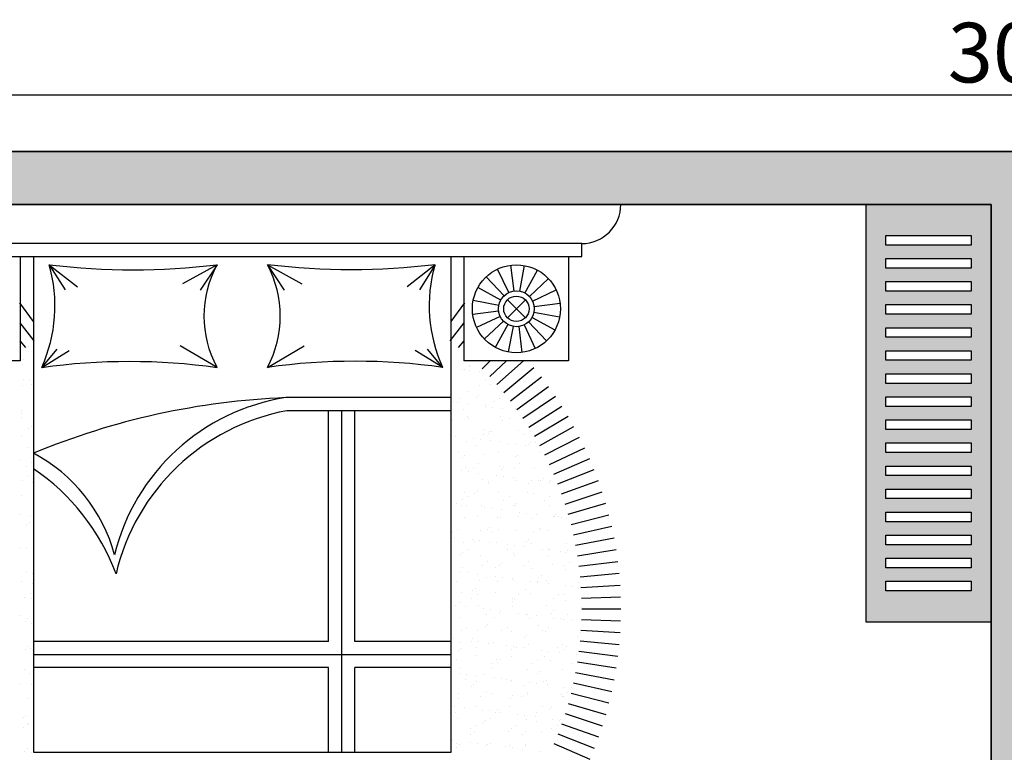
# Model space of a CAD drawing. Units: inches. Extents: x 1566 to 2546, y 1087 to 2705.
# Tile 22 of 27: x 2130 to 2278, y 1694 to 1804. Entities that reach past the tile are written whole.
import ezdxf

# ---------------------------------------------------------------- set-up
doc = ezdxf.new("R2010")
doc.units = ezdxf.units.IN
for name, color, linetype, lineweight in [('A-ANNO-DIMS', 2, 'Continuous', 18), ('A-FURN', 8, 'Continuous', 18), ('A-WALL', 7, 'Continuous', 35), ('A-WALL-PATT', 8, 'Continuous', 13)]:
    doc.layers.add(name, color=color, linetype=linetype, lineweight=lineweight)
for name, color, linetype in [('A-FRN', 11, 'Continuous'), ('A-HT', 15, 'Continuous'), ('L-HT', 1, 'Continuous'), ('MESA', 7, 'Continuous')]:
    doc.layers.add(name, color=color, linetype=linetype)
doc.styles.get("Standard").update_dxf_attribs({"font": 'arial.ttf'})
doc.dimstyles.new('ISO-25', dxfattribs={"dimtxt": 2.5, "dimasz": 2.5, "dimexe": 1.25, "dimexo": 0.625, "dimtad": 1, "dimtxsty": 'Standard', "dimcen": 2.5, "dimadec": 0, "dimazin": 0, "dimtfac": 1, "dimtmove": 0, "dimatfit": 3, "dimfxl": 1, "dimarcsym": 0})

# ---------------------------------------------------------------- blocks, each defined once
blk = doc.blocks.new('*D2')
at = {"layer": 'A-ANNO-DIMS', "color": 0, "lineweight": -2, "transparency": 16777216}
for p, q in [((2098.29, 1785.06), (2098.29, 1794.2)), ((2458.29, 1785.06), (2458.29, 1794.2)), ((2100.79, 1792.95), (2455.79, 1792.95))]:
    blk.add_line(p, q, dxfattribs=at)
at = {"layer": 'A-ANNO-DIMS', "color": 0, "transparency": 16777216}
for points in [[(2100.79, 1793.37), (2100.79, 1792.53), (2098.29, 1792.95)], [(2455.79, 1793.37), (2455.79, 1792.53), (2458.29, 1792.95)]]:
    blk.add_solid(points, dxfattribs=at)
at = {"layer": 'Defpoints', "color": 0, "transparency": 16777216}
for p in [(2458.29, 1792.95), (2098.29, 1784.43), (2458.29, 1784.43)]:
    blk.add_point(p, dxfattribs=at)
at = {"layer": 'A-ANNO-DIMS', "color": 0, "transparency": 16777216, "insert": (2278.29, 1798.17), "char_height": 9, "attachment_point": 5}
blk.add_mtext("30'", dxfattribs=at)
blk = doc.blocks.new('*X21')
at = {"color": 0}
for p, q in [((1.1667, 2.0955), (1.1667, 2.0955)), ((1.1756, 2.0872), (1.1756, 2.0872)), ((1.1927, 2.0989), (1.1927, 2.0989)), ((2.8216, 2.08), (2.8216, 2.08)), ((3.0086, 2.079), (3.0086, 2.079)), ((3.0247, 2.0756), (3.0247, 2.0756)), ((3.0346, 2.0825), (3.0346, 2.0825)), ((3.0752, 2.0878), (3.0752, 2.0878)), ((3.1432, 2.0968), (3.1432, 2.0968)), ((2.8061, 2.0524), (2.8061, 2.0524)), ((2.8215, 2.0663), (2.8215, 2.0663)), ((2.8309, 2.0716), (2.8309, 2.0716)), ((2.874, 2.0613), (2.874, 2.0613)), ((2.9, 2.0647), (2.9, 2.0647)), ((2.9303, 2.0732), (2.9303, 2.0732)), ((2.9407, 2.0701), (2.9407, 2.0701)), ((2.9494, 2.0657), (2.9494, 2.0657)), ((3.0845, 2.0705), (3.0845, 2.0705)), ((3.086, 2.0735), (3.086, 2.0735)), ((1.1609, 2.0067), (1.1609, 2.0067)), ((2.8737, 2.0098), (2.8737, 2.0098)), ((2.8744, 2.0317), (2.8744, 2.0317)), ((2.8891, 2.0194), (2.8891, 2.0194)), ((3.02, 2.0211), (3.02, 2.0211)), ((3.0294, 2.0101), (3.0294, 2.0101)), ((3.0744, 2.03), (3.0744, 2.03)), ((3.0837, 2.0216), (3.0837, 2.0216)), ((3.1479, 2.0205), (3.1479, 2.0205)), ((3.1851, 2.0104), (3.1851, 2.0104)), ((1.1614, 1.9668), (1.1614, 1.9668)), ((1.1788, 1.9909), (1.1788, 1.9909)), ((1.182, 1.9932), (1.182, 1.9932)), ((2.8247, 1.9699), (2.8247, 1.9699)), ((2.8947, 1.9964), (2.8947, 1.9964)), ((2.9241, 1.9861), (2.9241, 1.9861)), ((2.9333, 1.9777), (2.9333, 1.9777)), ((2.9526, 1.9693), (2.9526, 1.9693)), ((3.0505, 1.9966), (3.0505, 1.9966)), ((3.0876, 1.9742), (3.0876, 1.9742)), ((3.1213, 1.9644), (3.1213, 1.9644)), ((3.1272, 1.9817), (3.1272, 1.9817)), ((3.1893, 1.9734), (3.1893, 1.9734)), ((3.2062, 1.9969), (3.2062, 1.9969)), ((3.2153, 1.9768), (3.2153, 1.9768)), ((3.2185, 1.9759), (3.2185, 1.9759)), ((1.1707, 1.9584), (1.1707, 1.9584)), ((2.8115, 1.9236), (2.8115, 1.9236)), ((2.8149, 1.9477), (2.8149, 1.9477)), ((2.8522, 1.929), (2.8522, 1.929)), ((2.9201, 1.9379), (2.9201, 1.9379)), ((2.9461, 1.9414), (2.9461, 1.9414)), ((2.9707, 1.948), (2.9707, 1.948)), ((2.9768, 1.9378), (2.9768, 1.9378)), ((2.9868, 1.9467), (2.9868, 1.9467)), ((3.0232, 1.9247), (3.0232, 1.9247)), ((3.0547, 1.9556), (3.0547, 1.9556)), ((3.0807, 1.9591), (3.0807, 1.9591)), ((3.1264, 1.9483), (3.1264, 1.9483)), ((3.1511, 1.9241), (3.1511, 1.9241)), ((3.1769, 1.9361), (3.1769, 1.9361)), ((3.1861, 1.9277), (3.1861, 1.9277)), ((1.1819, 1.8945), (1.1819, 1.8945)), ((2.8265, 1.894), (2.8265, 1.894)), ((2.8923, 1.9231), (2.8923, 1.9231)), ((3.0266, 1.8922), (3.0266, 1.8922)), ((3.2296, 1.8878), (3.2296, 1.8878)), ((2.8278, 1.8736), (2.8278, 1.8736)), ((2.8763, 1.8484), (2.8763, 1.8484)), ((2.914, 1.8846), (2.914, 1.8846)), ((2.9351, 1.8712), (2.9351, 1.8712)), ((2.9557, 1.873), (2.9557, 1.873)), ((3.0358, 1.8838), (3.0358, 1.8838)), ((3.0697, 1.8849), (3.0697, 1.8849)), ((3.0908, 1.8779), (3.0908, 1.8779)), ((3.0908, 1.8714), (3.0908, 1.8714)), ((3.2217, 1.8795), (3.2217, 1.8795)), ((3.2255, 1.8852), (3.2255, 1.8852)), ((3.2354, 1.85), (3.2354, 1.85)), ((3.2465, 1.8717), (3.2465, 1.8717)), ((3.2614, 1.8534), (3.2614, 1.8534)), ((1.1504, 1.8344), (1.1504, 1.8344)), ((1.191, 1.8397), (1.191, 1.8397)), ((2.8553, 1.8225), (2.8553, 1.8225)), ((2.8855, 1.8399), (2.8855, 1.8399)), ((2.8954, 1.8267), (2.8954, 1.8267)), ((2.9662, 1.8145), (2.9662, 1.8145)), ((2.9922, 1.818), (2.9922, 1.818)), ((3.011, 1.8228), (3.011, 1.8228)), ((3.0263, 1.8284), (3.0263, 1.8284)), ((3.0329, 1.8233), (3.0329, 1.8233)), ((3.0793, 1.8439), (3.0793, 1.8439)), ((3.1008, 1.8323), (3.1008, 1.8323)), ((3.1268, 1.8357), (3.1268, 1.8357)), ((3.1542, 1.8278), (3.1542, 1.8278)), ((3.1667, 1.8231), (3.1667, 1.8231)), ((3.1674, 1.841), (3.1674, 1.841)), ((1.1663, 1.7807), (1.1663, 1.7807)), ((1.1851, 1.7982), (1.1851, 1.7982)), ((2.831, 1.7773), (2.831, 1.7773)), ((2.8316, 1.7968), (2.8316, 1.7968)), ((2.8576, 1.8002), (2.8576, 1.8002)), ((2.8983, 1.8056), (2.8983, 1.8056)), ((2.929, 1.8), (2.929, 1.8)), ((2.9589, 1.7766), (2.9589, 1.7766)), ((3.0939, 1.7815), (3.0939, 1.7815)), ((3.1291, 1.7983), (3.1291, 1.7983)), ((3.1383, 1.7899), (3.1383, 1.7899)), ((3.2248, 1.7832), (3.2248, 1.7832)), ((2.8198, 1.7457), (2.8198, 1.7457)), ((2.9544, 1.7594), (2.9544, 1.7594)), ((2.9755, 1.7459), (2.9755, 1.7459)), ((2.9788, 1.7544), (2.9788, 1.7544)), ((2.988, 1.746), (2.988, 1.746)), ((3.1101, 1.7597), (3.1101, 1.7597)), ((3.1312, 1.7462), (3.1312, 1.7462)), ((3.1818, 1.75), (3.1818, 1.75)), ((3.2658, 1.7599), (3.2658, 1.7599)), ((1.1704, 1.7076), (1.1704, 1.7076)), ((1.1882, 1.7018), (1.1882, 1.7018)), ((1.1965, 1.711), (1.1965, 1.711)), ((2.8285, 1.7106), (2.8285, 1.7106)), ((2.8377, 1.7021), (2.8377, 1.7021)), ((2.8957, 1.6973), (2.8957, 1.6973)), ((2.8986, 1.7304), (2.8986, 1.7304)), ((3.0295, 1.7321), (3.0295, 1.7321)), ((3.0315, 1.7061), (3.0315, 1.7061)), ((3.0514, 1.6976), (3.0514, 1.6976)), ((3.079, 1.6999), (3.079, 1.6999)), ((3.1469, 1.7089), (3.1469, 1.7089)), ((3.1574, 1.7314), (3.1574, 1.7314)), ((3.1729, 1.7123), (3.1729, 1.7123)), ((3.2071, 1.6979), (3.2071, 1.6979)), ((3.2135, 1.7176), (3.2135, 1.7176)), ((3.2316, 1.7044), (3.2316, 1.7044)), ((3.2815, 1.7266), (3.2815, 1.7266)), ((1.1829, 1.6942), (1.1829, 1.6942)), ((2.8098, 1.6645), (2.8098, 1.6645)), ((2.8341, 1.6809), (2.8341, 1.6809)), ((2.8777, 1.6734), (2.8777, 1.6734)), ((2.8812, 1.6623), (2.8812, 1.6623)), ((2.9037, 1.6769), (2.9037, 1.6769)), ((2.9444, 1.6822), (2.9444, 1.6822)), ((2.962, 1.6803), (2.962, 1.6803)), ((3.0123, 1.6911), (3.0123, 1.6911)), ((3.0383, 1.6946), (3.0383, 1.6946)), ((3.0813, 1.6605), (3.0813, 1.6605)), ((3.0971, 1.6852), (3.0971, 1.6852)), ((3.228, 1.6868), (3.228, 1.6868)), ((3.2408, 1.696), (3.2408, 1.696)), ((2.8391, 1.6339), (2.8391, 1.6339)), ((2.9017, 1.634), (2.9017, 1.634)), ((2.9948, 1.6342), (2.9948, 1.6342)), ((3.0326, 1.6357), (3.0326, 1.6357)), ((3.0905, 1.6521), (3.0905, 1.6521)), ((3.1505, 1.6345), (3.1505, 1.6345)), ((3.1605, 1.6351), (3.1605, 1.6351)), ((3.2843, 1.6561), (3.2843, 1.6561)), ((3.2956, 1.64), (3.2956, 1.64)), ((1.1683, 1.5973), (1.1683, 1.5973)), ((1.1775, 1.5889), (1.1775, 1.5889)), ((1.1914, 1.6055), (1.1914, 1.6055)), ((2.8373, 1.5846), (2.8373, 1.5846)), ((2.8602, 1.6205), (2.8602, 1.6205)), ((2.931, 1.6167), (2.931, 1.6167)), ((2.9402, 1.6082), (2.9402, 1.6082)), ((2.9652, 1.584), (2.9652, 1.584)), ((3.0159, 1.6207), (3.0159, 1.6207)), ((3.1002, 1.5888), (3.1002, 1.5888)), ((3.134, 1.6122), (3.134, 1.6122)), ((3.1716, 1.621), (3.1716, 1.621)), ((3.193, 1.5855), (3.193, 1.5855)), ((3.219, 1.5889), (3.219, 1.5889)), ((3.2311, 1.5905), (3.2311, 1.5905)), ((3.2596, 1.5943), (3.2596, 1.5943)), ((1.1486, 1.5753), (1.1486, 1.5753)), ((2.9238, 1.55), (2.9238, 1.55)), ((2.9361, 1.5721), (2.9361, 1.5721)), ((2.9498, 1.5535), (2.9498, 1.5535)), ((2.9837, 1.5683), (2.9837, 1.5683)), ((2.9905, 1.5588), (2.9905, 1.5588)), ((3.0584, 1.5678), (3.0584, 1.5678)), ((3.0844, 1.5712), (3.0844, 1.5712)), ((3.0918, 1.5724), (3.0918, 1.5724)), ((3.1251, 1.5765), (3.1251, 1.5765)), ((3.1838, 1.5666), (3.1838, 1.5666)), ((3.193, 1.5582), (3.193, 1.5582)), ((3.2475, 1.5727), (3.2475, 1.5727)), ((1.1945, 1.5091), (1.1945, 1.5091)), ((2.8152, 1.5357), (2.8152, 1.5357)), ((2.8334, 1.5245), (2.8334, 1.5245)), ((2.8559, 1.5411), (2.8559, 1.5411)), ((2.8795, 1.5087), (2.8795, 1.5087)), ((2.9049, 1.5377), (2.9049, 1.5377)), ((3.0334, 1.5227), (3.0334, 1.5227)), ((3.0352, 1.509), (3.0352, 1.509)), ((3.0358, 1.5394), (3.0358, 1.5394)), ((3.0427, 1.5143), (3.0427, 1.5143)), ((3.1637, 1.5388), (3.1637, 1.5388)), ((3.1909, 1.5093), (3.1909, 1.5093)), ((3.2365, 1.5183), (3.2365, 1.5183)), ((3.2987, 1.5436), (3.2987, 1.5436)), ((1.1667, 1.5056), (1.1667, 1.5056)), ((1.1878, 1.4921), (1.1878, 1.4921)), ((2.8404, 1.4882), (2.8404, 1.4882)), ((2.8831, 1.4789), (2.8831, 1.4789)), ((2.9006, 1.4953), (2.9006, 1.4953)), ((2.9683, 1.4876), (2.9683, 1.4876)), ((3.0563, 1.4955), (3.0563, 1.4955)), ((3.0862, 1.4744), (3.0862, 1.4744)), ((3.1034, 1.4925), (3.1034, 1.4925)), ((3.212, 1.4958), (3.212, 1.4958)), ((3.2343, 1.4942), (3.2343, 1.4942)), ((3.2862, 1.4727), (3.2862, 1.4727)), ((1.1541, 1.4465), (1.1541, 1.4465)), ((1.1947, 1.4519), (1.1947, 1.4519)), ((2.8208, 1.4466), (2.8208, 1.4466)), ((2.8924, 1.4704), (2.8924, 1.4704)), ((2.908, 1.4414), (2.908, 1.4414)), ((2.9765, 1.4469), (2.9765, 1.4469)), ((3.0366, 1.4354), (3.0366, 1.4354)), ((3.0389, 1.443), (3.0389, 1.443)), ((3.1045, 1.4444), (3.1045, 1.4444)), ((3.1305, 1.4478), (3.1305, 1.4478)), ((3.1322, 1.4472), (3.1322, 1.4472)), ((3.1668, 1.4424), (3.1668, 1.4424)), ((3.1712, 1.4532), (3.1712, 1.4532)), ((3.2391, 1.4621), (3.2391, 1.4621)), ((3.2651, 1.4655), (3.2651, 1.4655)), ((3.2879, 1.4475), (3.2879, 1.4475)), ((3.2954, 1.4643), (3.2954, 1.4643)), ((1.1732, 1.4112), (1.1732, 1.4112)), ((1.1977, 1.4128), (1.1977, 1.4128)), ((2.8353, 1.4089), (2.8353, 1.4089)), ((2.8613, 1.4124), (2.8613, 1.4124)), ((2.902, 1.4177), (2.902, 1.4177)), ((2.9359, 1.4306), (2.9359, 1.4306)), ((2.9699, 1.4267), (2.9699, 1.4267)), ((2.9959, 1.4301), (2.9959, 1.4301)), ((3.1065, 1.3961), (3.1065, 1.3961)), ((3.1359, 1.4288), (3.1359, 1.4288)), ((3.1451, 1.4204), (3.1451, 1.4204)), ((3.2374, 1.3978), (3.2374, 1.3978)), ((2.8436, 1.3919), (2.8436, 1.3919)), ((2.9199, 1.3835), (2.9199, 1.3835)), ((2.9409, 1.37), (2.9409, 1.37)), ((2.9715, 1.3913), (2.9715, 1.3913)), ((2.9856, 1.385), (2.9856, 1.385)), ((2.9948, 1.3765), (2.9948, 1.3765)), ((3.0756, 1.3838), (3.0756, 1.3838)), ((3.0967, 1.3703), (3.0967, 1.3703)), ((3.1886, 1.3805), (3.1886, 1.3805)), ((3.2313, 1.384), (3.2313, 1.384)), ((3.2524, 1.3706), (3.2524, 1.3706)), ((2.8353, 1.3411), (2.8353, 1.3411)), ((2.8445, 1.3326), (2.8445, 1.3326)), ((2.8611, 1.3214), (2.8611, 1.3214)), ((2.9112, 1.345), (2.9112, 1.345)), ((3.0169, 1.3217), (3.0169, 1.3217)), ((3.0383, 1.3367), (3.0383, 1.3367)), ((3.0421, 1.3467), (3.0421, 1.3467)), ((3.1506, 1.321), (3.1506, 1.321)), ((3.17, 1.3461), (3.17, 1.3461)), ((3.1726, 1.322), (3.1726, 1.322)), ((3.1766, 1.3244), (3.1766, 1.3244)), ((3.2173, 1.3298), (3.2173, 1.3298)), ((3.2384, 1.3349), (3.2384, 1.3349)), ((3.2476, 1.3265), (3.2476, 1.3265)), ((1.1484, 1.3183), (1.1484, 1.3183)), ((1.1741, 1.3197), (1.1741, 1.3197)), ((2.8467, 1.2956), (2.8467, 1.2956)), ((2.8814, 1.2855), (2.8814, 1.2855)), ((2.888, 1.2928), (2.888, 1.2928)), ((2.9074, 1.289), (2.9074, 1.289)), ((2.9481, 1.2943), (2.9481, 1.2943)), ((2.9746, 1.2949), (2.9746, 1.2949)), ((3.016, 1.3033), (3.016, 1.3033)), ((3.042, 1.3067), (3.042, 1.3067)), ((3.0827, 1.312), (3.0827, 1.312)), ((3.0881, 1.291), (3.0881, 1.291)), ((3.0973, 1.2826), (3.0973, 1.2826)), ((3.1097, 1.2998), (3.1097, 1.2998)), ((3.2406, 1.3015), (3.2406, 1.3015)), ((2.8045, 1.258), (2.8045, 1.258)), ((2.8135, 1.2766), (2.8135, 1.2766)), ((2.8256, 1.2446), (2.8256, 1.2446)), ((2.9143, 1.2487), (2.9143, 1.2487)), ((2.9378, 1.2472), (2.9378, 1.2472)), ((2.9602, 1.2583), (2.9602, 1.2583)), ((2.9813, 1.2448), (2.9813, 1.2448)), ((3.0452, 1.2503), (3.0452, 1.2503)), ((3.1159, 1.2586), (3.1159, 1.2586)), ((3.137, 1.2451), (3.137, 1.2451)), ((3.1731, 1.2497), (3.1731, 1.2497)), ((1.1751, 1.2278), (1.1751, 1.2278)), ((1.1843, 1.2194), (1.1843, 1.2194)), ((2.947, 1.2387), (2.947, 1.2387)), ((3.1408, 1.2427), (3.1408, 1.2427)), ((1.1523, 1.1874), (1.1523, 1.1874)), ((1.1887, 1.1931), (1.1887, 1.1931)), ((2.8499, 1.1992), (2.8499, 1.1992)), ((2.9015, 1.1962), (2.9015, 1.1962)), ((2.9778, 1.1986), (2.9778, 1.1986)), ((2.9905, 1.1989), (2.9905, 1.1989)), ((2.9942, 1.1709), (2.9942, 1.1709)), ((3.0572, 1.1965), (3.0572, 1.1965)), ((3.0621, 1.1799), (3.0621, 1.1799)), ((3.0881, 1.1833), (3.0881, 1.1833)), ((3.1128, 1.2035), (3.1128, 1.2035)), ((3.1288, 1.1887), (3.1288, 1.1887)), ((3.1906, 1.1971), (3.1906, 1.1971)), ((3.1967, 1.1976), (3.1967, 1.1976)), ((3.1998, 1.1887), (3.1998, 1.1887)), ((3.2129, 1.1968), (3.2129, 1.1968)), ((3.2227, 1.201), (3.2227, 1.201)), ((3.2437, 1.2051), (3.2437, 1.2051)), ((2.8189, 1.1479), (2.8189, 1.1479)), ((2.8402, 1.155), (2.8402, 1.155)), ((2.8449, 1.1328), (2.8449, 1.1328)), ((2.8596, 1.1532), (2.8596, 1.1532)), ((2.9175, 1.1523), (2.9175, 1.1523)), ((2.9275, 1.1622), (2.9275, 1.1622)), ((2.9535, 1.1656), (2.9535, 1.1656)), ((3.0006, 1.1331), (3.0006, 1.1331)), ((3.0403, 1.1533), (3.0403, 1.1533)), ((3.0484, 1.154), (3.0484, 1.154)), ((3.0495, 1.1448), (3.0495, 1.1448)), ((3.1563, 1.1334), (3.1563, 1.1334)), ((3.1763, 1.1534), (3.1763, 1.1534)), ((1.1532, 1.1162), (1.1532, 1.1162)), ((2.853, 1.1029), (2.853, 1.1029)), ((2.866, 1.1194), (2.866, 1.1194)), ((2.89, 1.1094), (2.89, 1.1094)), ((2.8992, 1.1009), (2.8992, 1.1009)), ((2.9809, 1.1023), (2.9809, 1.1023)), ((3.0217, 1.1196), (3.0217, 1.1196)), ((3.093, 1.105), (3.093, 1.105)), ((3.116, 1.1071), (3.116, 1.1071)), ((3.1774, 1.1199), (3.1774, 1.1199)), ((1.1578, 1.0586), (1.1578, 1.0586)), ((1.1984, 1.064), (1.1984, 1.064)), ((2.9206, 1.056), (2.9206, 1.056)), ((2.9419, 1.071), (2.9419, 1.071)), ((2.9427, 1.0611), (2.9427, 1.0611)), ((3.0515, 1.0577), (3.0515, 1.0577)), ((3.0976, 1.0713), (3.0976, 1.0713)), ((3.1082, 1.0565), (3.1082, 1.0565)), ((3.1342, 1.0599), (3.1342, 1.0599)), ((3.1428, 1.0594), (3.1428, 1.0594)), ((3.1749, 1.0653), (3.1749, 1.0653)), ((3.1794, 1.057), (3.1794, 1.057)), ((1.18, 1.0417), (1.18, 1.0417)), ((2.839, 1.0211), (2.839, 1.0211)), ((2.865, 1.0245), (2.865, 1.0245)), ((2.9057, 1.0298), (2.9057, 1.0298)), ((2.9736, 1.0388), (2.9736, 1.0388)), ((2.9996, 1.0422), (2.9996, 1.0422)), ((3.0403, 1.0475), (3.0403, 1.0475)), ((3.152, 1.0509), (3.152, 1.0509)), ((1.15, 0.9812), (1.15, 0.9812)), ((1.1725, 1.0045), (1.1725, 1.0045)), ((1.1936, 0.991), (1.1936, 0.991)), ((2.8562, 1.0065), (2.8562, 1.0065)), ((2.8853, 1.0076), (2.8853, 1.0076)), ((2.9064, 0.9942), (2.9064, 0.9942)), ((2.9841, 1.0059), (2.9841, 1.0059)), ((2.9925, 1.0155), (2.9925, 1.0155)), ((3.0017, 1.007), (3.0017, 1.007)), ((3.041, 1.0079), (3.041, 1.0079)), ((3.0621, 0.9944), (3.0621, 0.9944)), ((3.1191, 1.0108), (3.1191, 1.0108)), ((2.8266, 0.9455), (2.8266, 0.9455)), ((2.8421, 0.9716), (2.8421, 0.9716)), ((2.8514, 0.9631), (2.8514, 0.9631)), ((2.9238, 0.9597), (2.9238, 0.9597)), ((2.9823, 0.9458), (2.9823, 0.9458)), ((3.0452, 0.9672), (3.0452, 0.9672)), ((3.0547, 0.9613), (3.0547, 0.9613)), ((3.138, 0.9461), (3.138, 0.9461)), ((1.1779, 0.9318), (1.1779, 0.9318)), ((2.8593, 0.9102), (2.8593, 0.9102)), ((2.8949, 0.9233), (2.8949, 0.9233)), ((2.9518, 0.9064), (2.9518, 0.9064)), ((2.9872, 0.9096), (2.9872, 0.9096)), ((3.0197, 0.9154), (3.0197, 0.9154)), ((3.0457, 0.9188), (3.0457, 0.9188)), ((3.0864, 0.9242), (3.0864, 0.9242)), ((3.0949, 0.9216), (3.0949, 0.9216)), ((3.1041, 0.9131), (3.1041, 0.9131)), ((3.1223, 0.9144), (3.1223, 0.9144)), ((1.1531, 0.8848), (1.1531, 0.8848)), ((2.8172, 0.8887), (2.8172, 0.8887)), ((2.8851, 0.8977), (2.8851, 0.8977)), ((2.9111, 0.9011), (2.9111, 0.9011)), ((2.9257, 0.8824), (2.9257, 0.8824)), ((2.9446, 0.8777), (2.9446, 0.8777)), ((2.9468, 0.8689), (2.9468, 0.8689)), ((2.9538, 0.8692), (2.9538, 0.8692)), ((3.0814, 0.8827), (3.0814, 0.8827)), ((3.1025, 0.8692), (3.1025, 0.8692)), ((1.1819, 0.8583), (1.1819, 0.8583)), ((1.1912, 0.8499), (1.1912, 0.8499)), ((2.9269, 0.8633), (2.9269, 0.8633)), ((3.0578, 0.865), (3.0578, 0.865)), ((1.1542, 0.8172), (1.1542, 0.8172)), ((1.156, 0.7995), (1.156, 0.7995)), ((2.8035, 0.8253), (2.8035, 0.8253)), ((2.8625, 0.8138), (2.8625, 0.8138)), ((2.867, 0.8203), (2.867, 0.8203)), ((2.9904, 0.8132), (2.9904, 0.8132)), ((2.9973, 0.8294), (2.9973, 0.8294)), ((3.0227, 0.8206), (3.0227, 0.8206)), ((1.1563, 0.7885), (1.1563, 0.7885)), ((2.8104, 0.7569), (2.8104, 0.7569)), ((2.8227, 0.76), (2.8227, 0.76)), ((2.847, 0.7855), (2.847, 0.7855)), ((2.8633, 0.7653), (2.8633, 0.7653)), ((2.9301, 0.767), (2.9301, 0.767)), ((2.9312, 0.7743), (2.9312, 0.7743)), ((2.9572, 0.7777), (2.9572, 0.7777)), ((2.9661, 0.7572), (2.9661, 0.7572)), ((2.9979, 0.7831), (2.9979, 0.7831)), ((3.0471, 0.7838), (3.0471, 0.7838)), ((2.8314, 0.7435), (2.8314, 0.7435)), ((2.8656, 0.7175), (2.8656, 0.7175)), ((2.8968, 0.7399), (2.8968, 0.7399)), ((2.906, 0.7314), (2.906, 0.7314)), ((2.9871, 0.7437), (2.9871, 0.7437)), ((2.9935, 0.7169), (2.9935, 0.7169)), ((1.1594, 0.6922), (1.1594, 0.6922)), ((1.1946, 0.692), (1.1946, 0.692)), ((2.9073, 0.6951), (2.9073, 0.6951)), ((2.9495, 0.6916), (2.9495, 0.6916)), ((1.1615, 0.6707), (1.1615, 0.6707)), ((1.1868, 0.6723), (1.1868, 0.6723)), ((2.9094, 0.6419), (2.9094, 0.6419)), ((2.9332, 0.6706), (2.9332, 0.6706)), ((1.159, 0.6151), (1.159, 0.6151)), ((2.8427, 0.6332), (2.8427, 0.6332)), ((2.8507, 0.6317), (2.8507, 0.6317)), ((2.8688, 0.6366), (2.8688, 0.6366)), ((2.8688, 0.6212), (2.8688, 0.6212)), ((2.8718, 0.6183), (2.8718, 0.6183)), ((1.1626, 0.5958), (1.1626, 0.5958)), ((2.8013, 0.5694), (2.8013, 0.5694)), ((2.849, 0.6021), (2.849, 0.6021)), ((1.1816, 0.5439), (1.1816, 0.5439))]:
    blk.add_line(p, q, dxfattribs=at)
blk = doc.blocks.new('A$C6796526C')
at = {"layer": 'A-FRN'}
for p, q in [((0, 3), (2.9, 3)), ((2.75, 2.85), (0.15, 2.85)), ((2.75, 2.8), (2.75, 2.85)), ((0.15, 2.8), (2.75, 2.8)), ((0.6, 2.8), (0.6, 2.4)), ((2.3, 2.4), (2.3, 2.8)), ((2.7, 2.8), (2.7, 2.4)), ((0.6, 2.4), (0.2, 2.4)), ((2.7, 2.4), (2.3, 2.4))]:
    blk.add_line(p, q, dxfattribs=at)
blk.add_lwpolyline([(0.65, 2.8), (0.65, 0.9), (2.25, 0.9), (2.25, 2.8)], dxfattribs=at)
for points in [[(0.6821, 2.3755, 0.175461), (0.7109, 2.7686)], [(0.7109, 2.7686, 0.059544), (1.3533, 2.7686)], [(1.3533, 2.3755, -0.248743), (1.3533, 2.7686)], [(2.1891, 2.7686, -0.059544), (1.5467, 2.7686)], [(1.5467, 2.3755, 0.248743), (1.5467, 2.7686)], [(2.2179, 2.3755, -0.175461), (2.1891, 2.7686)], [(0.6821, 2.3755, -0.069628), (1.3533, 2.3755)], [(2.2179, 2.3755, 0.069628), (1.5467, 2.3755)], [(2.25, 2.2594), (1.6173, 2.2594, 0.303651), (0.9607, 1.6568, 0.210515), (0.65, 2.0462)]]:
    blk.add_lwpolyline(points, format="xyb", dxfattribs=at)
for radius in [0.1686, 0.0686]:
    blk.add_circle((2.5, 2.6), radius, dxfattribs=at)
for centre, radius, start, end in [((2.75, 3), 0.15, 270, 0), ((1.7313, -0.5592), 2.8209, 92.3174, 112.5397)]:
    blk.add_arc(centre, radius, start, end, dxfattribs=at)
at = {"layer": 'A-HT'}
for p, q in [((0.65, 2.5511), (0.5977, 2.6231)), ((2.25, 2.5511), (2.3023, 2.6231)), ((0.6532, 2.4772), (0.6, 2.5458)), ((2.2468, 2.4772), (2.3, 2.5458)), ((0.6213, 2.4517), (0.6, 2.4775)), ((2.2787, 2.4517), (2.3, 2.4775)), ((2.3692, 2.3692), (2.4, 2.4)), ((2.3977, 2.3399), (2.4616, 2.4)), ((2.4251, 2.3097), (2.5276, 2.4)), ((2.4517, 2.2787), (2.5672, 2.3743)), ((2.4772, 2.2468), (2.5957, 2.3387)), ((2.5017, 2.2141), (2.6231, 2.3023)), ((2.5252, 2.1807), (2.6493, 2.265)), ((2.5476, 2.1466), (2.6743, 2.2269)), ((2.569, 2.1118), (2.6981, 2.1881)), ((2.5892, 2.0763), (2.7206, 2.1485)), ((2.6083, 2.0402), (2.742, 2.1083)), ((2.6263, 2.0035), (2.762, 2.0674)), ((2.6431, 1.9663), (2.7807, 2.0259)), ((2.6587, 1.9286), (2.7982, 1.9838)), ((2.6731, 1.8904), (2.8143, 1.9412)), ((2.6864, 1.8517), (2.829, 1.8981)), ((2.6984, 1.8127), (2.8424, 1.8545)), ((2.7092, 1.7733), (2.8544, 1.8106)), ((2.7187, 1.7336), (2.8651, 1.7663)), ((2.727, 1.6936), (2.8743, 1.7217)), ((2.734, 1.6534), (2.8821, 1.6768)), ((2.7397, 1.6129), (2.8886, 1.6317)), ((2.7442, 1.5723), (2.8936, 1.5865)), ((2.7474, 1.5316), (2.8971, 1.541)), ((2.7494, 1.4908), (2.8993, 1.4955)), ((2.75, 1.45), (2.9, 1.45)), ((2.7494, 1.4092), (2.8993, 1.4045)), ((2.7474, 1.3684), (2.8971, 1.359)), ((2.7442, 1.3277), (2.8936, 1.3135)), ((2.7397, 1.2871), (2.8886, 1.2683)), ((2.734, 1.2466), (2.8821, 1.2232)), ((2.727, 1.2064), (2.8743, 1.1783)), ((2.7187, 1.1664), (2.8651, 1.1337)), ((2.7092, 1.1267), (2.8544, 1.0894)), ((2.6984, 1.0873), (2.8424, 1.0455)), ((2.6864, 1.0483), (2.829, 1.0019)), ((2.6731, 1.0096), (2.8143, 0.9588)), ((2.6587, 0.9714), (2.7982, 0.9162)), ((2.6431, 0.9337), (2.7807, 0.8741))]:
    blk.add_line(p, q, dxfattribs=at)
at = {"layer": 'L-HT'}
for p, q in [((0.7109, 2.7686), (0.8188, 2.6839)), ((0.7109, 2.7686), (0.7717, 2.6727)), ((1.3533, 2.7686), (1.2212, 2.6952)), ((1.3533, 2.7686), (1.2893, 2.6715)), ((1.5467, 2.7686), (1.6107, 2.6715)), ((1.5467, 2.7686), (1.6788, 2.6952)), ((2.1891, 2.7686), (2.0812, 2.6839)), ((2.1891, 2.7686), (2.1283, 2.6727)), ((2.4913, 2.668), (2.4786, 2.7672)), ((2.5127, 2.6674), (2.5313, 2.7656)), ((2.453, 2.6499), (2.3844, 2.7227)), ((2.4707, 2.662), (2.428, 2.7524)), ((2.5329, 2.6601), (2.581, 2.7478)), ((2.5499, 2.647), (2.6227, 2.7156)), ((2.4399, 2.6329), (2.3522, 2.681)), ((2.562, 2.6293), (2.6524, 2.672)), ((2.4326, 2.6127), (2.3344, 2.6313)), ((2.4657, 2.5657), (2.5343, 2.6343)), ((2.5343, 2.5657), (2.4657, 2.6343)), ((2.568, 2.6087), (2.6672, 2.6214)), ((2.432, 2.5913), (2.3328, 2.5786)), ((2.438, 2.5707), (2.3476, 2.528)), ((2.5601, 2.5671), (2.6478, 2.519)), ((2.5674, 2.5873), (2.6656, 2.5687)), ((2.4501, 2.553), (2.3773, 2.4844)), ((2.4671, 2.5399), (2.419, 2.4522)), ((2.4873, 2.5326), (2.4687, 2.4344)), ((2.5087, 2.532), (2.5214, 2.4328)), ((2.5293, 2.538), (2.572, 2.4476)), ((2.547, 2.5501), (2.6156, 2.4773)), ((1.3533, 2.3755), (1.2125, 2.4585)), ((1.5467, 2.3755), (1.6875, 2.4585)), ((0.6821, 2.3755), (0.7405, 2.4447)), ((0.6821, 2.3755), (0.7872, 2.4395)), ((2.2179, 2.3755), (2.1128, 2.4395)), ((2.2179, 2.3755), (2.1595, 2.4447)), ((2.25, 2.2094), (1.6212, 2.2094)), ((1.7809, 1.3249), (1.7809, 2.2094)), ((1.8309, 0.9), (1.8309, 2.2094)), ((1.8809, 1.3249), (1.8809, 2.2094)), ((1.7809, 1.3249), (0.65, 1.3249)), ((2.25, 1.3249), (1.8809, 1.3249)), ((0.65, 1.2749), (2.25, 1.2749)), ((1.7809, 1.2249), (0.65, 1.2249)), ((1.7809, 0.9), (1.7809, 1.2249)), ((1.8809, 0.9), (1.8809, 1.2249)), ((2.25, 1.2249), (1.8809, 1.2249))]:
    blk.add_line(p, q, dxfattribs=at)
blk.add_circle((2.5, 2.6), 0.0486, dxfattribs=at)
for centre, radius, start, end in [((1.7721, 1.396), 0.8272, 100.5107, 166.872), ((0.1786, 1.2908), 0.8406, 20.4105, 55.8901)]:
    blk.add_arc(centre, radius, start, end, dxfattribs=at)
at = {"layer": 'A-HT', "extrusion": (0, 0, -1), "zscale": -1, "rotation": 180}
blk.add_blockref('*X21', (0.55, 3), dxfattribs=at)
blk = doc.blocks.new('Banco Lintz')
at = {"layer": 'MESA', "ltscale": 0.05}
h = blk.add_hatch(color=256, dxfattribs=at)
h.dxf.hatch_style = 1
h.set_gradient(color1=(138, 84, 66), color2=(0, 0, 0), one_color=1, name='INVCYLINDER')
h.paths.add_polyline_path([(0.48, 0), (0, 0), (0, -1.6), (0.48, -1.6)])
h.paths.add_polyline_path([(0.4034, -0.5091), (0.0766, -0.5091), (0.0766, -0.4724), (0.4034, -0.4724)], flags=16)
h.paths.add_polyline_path([(0.4034, -0.5608), (0.4034, -0.5974), (0.0766, -0.5974), (0.0766, -0.5608)], flags=16)
h.paths.add_polyline_path([(0.4034, -0.4207), (0.0766, -0.4207), (0.0766, -0.384), (0.4034, -0.384)], flags=16)
h.paths.add_polyline_path([(0.4034, -0.6491), (0.4034, -0.6858), (0.0766, -0.6858), (0.0766, -0.6491)], flags=16)
h.paths.add_polyline_path([(0.4034, -0.3323), (0.0766, -0.3323), (0.0766, -0.2957), (0.4034, -0.2957)], flags=16)
h.paths.add_polyline_path([(0.4034, -0.7375), (0.4034, -0.7741), (0.0766, -0.7741), (0.0766, -0.7375)], flags=16)
h.paths.add_polyline_path([(0.4034, -0.244), (0.0766, -0.244), (0.0766, -0.2073), (0.4034, -0.2073)], flags=16)
h.paths.add_polyline_path([(0.4034, -0.8259), (0.4034, -0.8625), (0.0766, -0.8625), (0.0766, -0.8259)], flags=16)
h.paths.add_polyline_path([(0.4034, -0.1556), (0.0766, -0.1556), (0.0766, -0.119), (0.4034, -0.119)], flags=16)
h.paths.add_polyline_path([(0.4034, -0.9142), (0.4034, -0.9509), (0.0766, -0.9509), (0.0766, -0.9142)], flags=16)
h.paths.add_polyline_path([(0.4034, -1.0026), (0.4034, -1.0392), (0.0766, -1.0392), (0.0766, -1.0026)], flags=16)
h.paths.add_polyline_path([(0.4034, -1.0909), (0.4034, -1.1276), (0.0766, -1.1276), (0.0766, -1.0909)], flags=16)
h.paths.add_polyline_path([(0.4034, -1.1793), (0.4034, -1.216), (0.0766, -1.216), (0.0766, -1.1793)], flags=16)
h.paths.add_polyline_path([(0.4034, -1.2677), (0.4034, -1.3043), (0.0766, -1.3043), (0.0766, -1.2677)], flags=16)
h.paths.add_polyline_path([(0.4034, -1.356), (0.4034, -1.3927), (0.0766, -1.3927), (0.0766, -1.356)], flags=16)
h.paths.add_polyline_path([(0.4034, -1.4444), (0.4034, -1.481), (0.0766, -1.481), (0.0766, -1.4444)], flags=16)
for points in [[(0, -1.6), (0.48, -1.6), (0.48, 0), (0, 0)], [(0.0766, -0.119), (0.4034, -0.119), (0.4034, -0.1556), (0.0766, -0.1556)], [(0.0766, -0.2073), (0.4034, -0.2073), (0.4034, -0.244), (0.0766, -0.244)], [(0.0766, -0.2957), (0.4034, -0.2957), (0.4034, -0.3323), (0.0766, -0.3323)], [(0.0766, -0.384), (0.4034, -0.384), (0.4034, -0.4207), (0.0766, -0.4207)], [(0.0766, -0.4724), (0.4034, -0.4724), (0.4034, -0.5091), (0.0766, -0.5091)], [(0.0766, -0.5608), (0.4034, -0.5608), (0.4034, -0.5974), (0.0766, -0.5974)], [(0.0766, -0.6491), (0.4034, -0.6491), (0.4034, -0.6858), (0.0766, -0.6858)], [(0.0766, -0.7375), (0.4034, -0.7375), (0.4034, -0.7741), (0.0766, -0.7741)], [(0.0766, -0.8259), (0.4034, -0.8259), (0.4034, -0.8625), (0.0766, -0.8625)], [(0.0766, -0.9142), (0.4034, -0.9142), (0.4034, -0.9509), (0.0766, -0.9509)], [(0.0766, -1.0026), (0.4034, -1.0026), (0.4034, -1.0392), (0.0766, -1.0392)], [(0.0766, -1.0909), (0.4034, -1.0909), (0.4034, -1.1276), (0.0766, -1.1276)], [(0.0766, -1.1793), (0.4034, -1.1793), (0.4034, -1.216), (0.0766, -1.216)], [(0.0766, -1.2677), (0.4034, -1.2677), (0.4034, -1.3043), (0.0766, -1.3043)], [(0.0766, -1.356), (0.4034, -1.356), (0.4034, -1.3927), (0.0766, -1.3927)], [(0.0766, -1.4444), (0.4034, -1.4444), (0.4034, -1.481), (0.0766, -1.481)]]:
    blk.add_lwpolyline(points, close=True, dxfattribs=at)

msp = doc.modelspace()

# ---------------------------------------------------------------- hatches: boundary and pattern name
at = {"layer": 'A-WALL-PATT'}
h = msp.add_hatch(color=256, dxfattribs=at)
h.dxf.hatch_style = 1
h.paths.add_polyline_path([(2106.29, 1385.43), (2228.29, 1385.43), (2228.29, 1391.43), (2224.29, 1391.43), (2224.29, 1389.43), (2106.29, 1389.43), (2106.29, 1402.93), (2098.29, 1402.93), (2098.29, 1343.43), (2106.29, 1343.43), (2106.29, 1347.74)], flags=17)
h.paths.add_polyline_path([(2106.29, 1259.43), (2098.29, 1259.43), (2098.29, 1209.43), (2155.29, 1209.43), (2155.29, 1217.43), (2143.41, 1217.43), (2106.29, 1217.43)], flags=17)
h.paths.add_polyline_path([(2334.29, 1217.43), (2280.29, 1217.43), (2280.29, 1389.43), (2284.29, 1389.43), (2284.29, 1391.43), (2284.29, 1393.43), (2276.29, 1393.43), (2276.29, 1217.43), (2227.29, 1217.43), (2227.29, 1209.43), (2334.29, 1209.43)], flags=17)
h.paths.add_polyline_path([(2106.29, 1486.43), (2098.29, 1486.43), (2098.29, 1460.88), (2099.11, 1461.64), (2100.44, 1462.65), (2101.57, 1463.26), (2099.97, 1460.62), (2098.29, 1458.1), (2098.29, 1456.93), (2100.35, 1456.93), (2100.77, 1457.12), (2103.56, 1457.95), (2106.29, 1458.4), (2106.29, 1470.43), (2224.29, 1470.43), (2224.29, 1427.43), (2228.29, 1427.43), (2228.29, 1474.43), (2192.29, 1474.43), (2192.29, 1476.43), (2188.29, 1476.43), (2188.29, 1474.43), (2106.29, 1474.43)], flags=17)
h.paths.add_polyline_path([(2106.29, 1585.43), (2192.29, 1585.43), (2192.29, 1589.43), (2098.29, 1589.43), (2098.29, 1573.93), (2106.29, 1573.93)], flags=17)
h.paths.add_polyline_path([(2228.29, 1585.43), (2232.29, 1585.43), (2232.29, 1589.43), (2224.29, 1589.43), (2222.29, 1589.43), (2222.29, 1585.43), (2224.29, 1585.43), (2224.29, 1532.43), (2106.29, 1532.43), (2106.29, 1543.93), (2098.29, 1543.93), (2098.29, 1516.43), (2106.29, 1516.43), (2106.29, 1528.43), (2188.29, 1528.43), (2188.29, 1506.43), (2192.29, 1506.43), (2192.29, 1528.43), (2224.29, 1528.43), (2224.29, 1506.43), (2228.29, 1506.43)], flags=17)
h.paths.add_polyline_path([(2106.29, 1680.43), (2098.29, 1680.43), (2098.29, 1625.43), (2106.29, 1625.43)], flags=17)
h.paths.add_polyline_path([(2458.29, 1784.43), (2098.29, 1784.43), (2098.29, 1776.43), (2276.29, 1776.43), (2276.29, 1589.43), (2268.29, 1589.43), (2268.29, 1585.43), (2280.29, 1585.43), (2280.29, 1652.43), (2284.29, 1652.43), (2284.29, 1656.43), (2280.29, 1656.43), (2280.29, 1776.43), (2398.29, 1776.43), (2398.29, 1746.43), (2402.29, 1746.43), (2402.29, 1776.43), (2450.29, 1776.43), (2450.29, 1532.43), (2375.49, 1532.43), (2328.29, 1532.43), (2328.29, 1612.43), (2324.29, 1612.43), (2324.29, 1528.43), (2450.29, 1528.43), (2450.29, 1447.43), (2291.29, 1447.43), (2291.29, 1443.43), (2324.29, 1443.43), (2324.29, 1393.43), (2320.29, 1393.43), (2320.29, 1389.43), (2330.29, 1389.43), (2330.29, 1393.43), (2328.29, 1393.43), (2328.29, 1443.43), (2412.29, 1443.43), (2412.29, 1433.43), (2416.29, 1433.43), (2416.29, 1443.43), (2450.29, 1443.43), (2450.29, 1393.43), (2416.29, 1393.43), (2416.29, 1403.43), (2412.29, 1403.43), (2412.29, 1393.43), (2360.29, 1393.43), (2360.29, 1389.43), (2450.29, 1389.43), (2450.29, 1217.43), (2396.29, 1217.43), (2396.29, 1209.43), (2450.29, 1209.43), (2450.29, 1136.43), (2458.29, 1136.43)])

# ---------------------------------------------------------------- linework, layer by layer
at = {"layer": 'A-WALL'}
for p, q in [((2098.29, 1784.43), (2458.29, 1784.43)), ((2098.29, 1776.43), (2276.29, 1776.43)), ((2276.29, 1589.43), (2276.29, 1776.43))]:
    msp.add_line(p, q, dxfattribs=at)

# ---------------------------------------------------------------- block references
at = {"layer": 'A-FURN', "xscale": 39.3701, "yscale": 39.3701, "zscale": 39.3701}
for name, p in [('A$C6796526C', (2106.29, 1658.32)), ('Banco Lintz', (2257.39, 1776.43))]:
    msp.add_blockref(name, p, dxfattribs=at)

# ---------------------------------------------------------------- dimensions: what is measured, and where the dimension line sits
at = {"layer": 'A-ANNO-DIMS'}
dim = msp.add_linear_dim(base=(2458.29, 1792.95), p1=(2098.29, 1784.43), p2=(2458.29, 1784.43), dimstyle='ISO-25', override={"dimtxt": 9, "dimdec": 1, "dimlunit": 3, "dimclrd": 0, "dimclre": 0, "dimclrt": 0, "dimtdec": 1, "dimtmove": 1}, dxfattribs=at)
dim.commit()
dim.dimension.update_dxf_attribs({"geometry": '*D2', "text_midpoint": (2278.29, 1798.17)})

doc.saveas('drawing.dxf')
